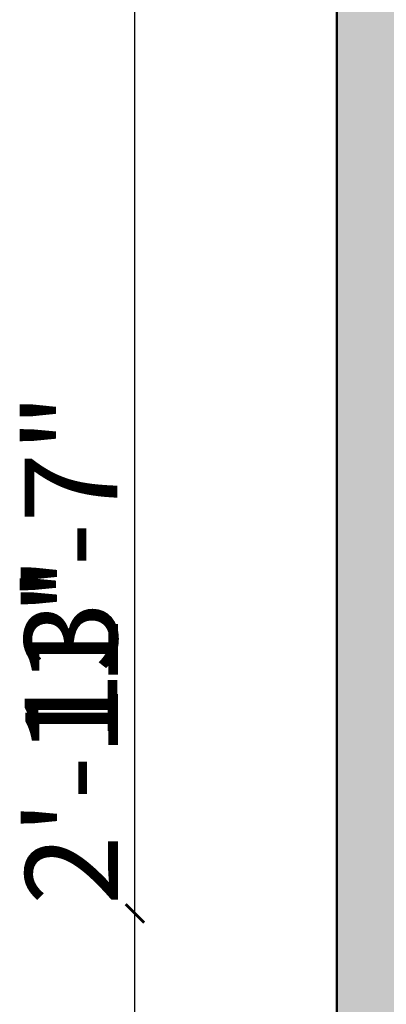
# Model space of a CAD drawing. Units: inches. Extents: x 2419 to 2878, y 1068 to 1713.
# Tile 1 of 20: x 2429 to 2478, y 1153 to 1286. Entities that reach past the tile are written whole.
import ezdxf

# ---------------------------------------------------------------- set-up
doc = ezdxf.new("R2010")
doc.units = ezdxf.units.IN
doc.layers.add('A-ANNO-DIMS', color=2, linetype='Continuous', lineweight=18)
doc.layers.add('A-WALL', color=7, linetype='Continuous', lineweight=50)
doc.layers.add('A-WALL-PATT', color=18, linetype='Continuous', lineweight=13, true_color=0x000000)
doc.styles.get("Standard").update_dxf_attribs({"font": 'arial.ttf'})
doc.dimstyles.new('ISO-25', dxfattribs={"dimtxt": 12.5, "dimasz": 2.5, "dimexe": 1.25, "dimexo": 0.625, "dimtad": 1, "dimdec": 0, "dimlunit": 4, "dimtxsty": 'Standard', "dimblk": 'ARCHTICK', "dimcen": 2.5, "dimse1": 1, "dimse2": 1, "dimclrd": 4, "dimadec": 0, "dimazin": 0, "dimtfac": 1, "dimtdec": 0, "dimtmove": 0, "dimatfit": 3, "dimfxl": 1, "dimarcsym": 0})

# ---------------------------------------------------------------- blocks, each defined once
blk = doc.blocks.new('_ArchTick')
at = {"color": 0, "linetype": 'ByBlock', "const_width": 0.15}
blk.add_lwpolyline([(-0.5, -0.5), (0.5, 0.5)], dxfattribs=at)
blk = doc.blocks.new('*D38')
at = {"layer": 'A-ANNO-DIMS', "color": 4, "lineweight": -2, "transparency": 16777216}
for p, q in [((2444.314464000002, 1165.602617), (2444.314464000002, 1212.505754789905)), ((2444.314464000002, 1130.812987), (2444.314464000002, 1165.602617))]:
    blk.add_line(p, q, dxfattribs=at)
at = {"layer": 'Defpoints', "color": 0, "transparency": 16777216}
for p in [(2444.314464000002, 1165.602617), (2656.740829000001, 1165.602617), (2656.740829000001, 1130.812987)]:
    blk.add_point(p, dxfattribs=at)
at = {"layer": 'A-ANNO-DIMS', "color": 4, "lineweight": -2, "transparency": 16777216, "xscale": 2.5, "yscale": 2.5, "zscale": 2.5}
for p, rotation in [((2444.314464000002, 1165.602617), 90), ((2444.314464000002, 1130.812987), 270)]:
    blk.add_blockref('_ArchTick', p, dxfattribs=dict(at, rotation=rotation))
at = {"layer": 'A-ANNO-DIMS', "color": 0, "transparency": 16777216, "insert": (2437.413884190998, 1190.304185894951), "char_height": 12.5, "attachment_point": 5, "rotation": 90}
blk.add_mtext('2\'-11"', dxfattribs=at)
blk = doc.blocks.new('*D54')
at = {"layer": 'A-ANNO-DIMS', "color": 4, "lineweight": -2, "transparency": 16777216}
blk.add_line((2444.314464000002, 1130.812987), (2444.314464000002, 1293.812987), dxfattribs=at)
at = {"layer": 'Defpoints', "color": 0, "transparency": 16777216}
for p in [(2444.314464000002, 1293.812987), (2480.514464000001, 1293.812987), (2480.514464000001, 1130.812987)]:
    blk.add_point(p, dxfattribs=at)
at = {"layer": 'A-ANNO-DIMS', "color": 4, "lineweight": -2, "transparency": 16777216, "xscale": 2.5, "yscale": 2.5, "zscale": 2.5}
for p, rotation in [((2444.314464000002, 1293.812987), 90), ((2444.314464000002, 1130.812987), 270)]:
    blk.add_blockref('_ArchTick', p, dxfattribs=dict(at, rotation=rotation))
at = {"layer": 'A-ANNO-DIMS', "color": 0, "transparency": 16777216, "insert": (2437.30303835198, 1212.312987), "char_height": 12.5, "attachment_point": 5, "rotation": 90}
blk.add_mtext('13\'-7"', dxfattribs=at)

msp = doc.modelspace()

# ---------------------------------------------------------------- hatches: boundary and pattern name
at = {"layer": 'A-WALL-PATT'}
h = msp.add_hatch(color=256, dxfattribs=at)
h.dxf.hatch_style = 1
h.paths.add_polyline_path([(2780.514463761465, 1577.812987234935), (2471.514463761465, 1577.812987234935), (2471.514463761465, 1121.812987234935), (2780.514463761465, 1121.812987234935)])
h.paths.add_polyline_path([(2480.514463761465, 1568.812987234935), (2771.514463761465, 1568.812987234935), (2771.514463761465, 1130.812987234935), (2480.514463761465, 1130.812987234935)], flags=16)
h.paths.add_polyline_path([(2528.514463761465, 1568.812987234935), (2528.514463761465, 1512.812987234935), (2594.514463761465, 1512.812987234935), (2594.514463761465, 1414.812987234935), (2596.568399739099, 1414.812987234935), (2596.568399739099, 1441.609368546496), (2597.816088158561, 1441.609368546496), (2597.816088158561, 1441.582062289591, -0.38401605427067), (2625.03494332709, 1414.812987234935), (2725.514463761465, 1414.812987234935), (2725.514463761465, 1567.54501314674), (2728.302225194595, 1567.54501314674), (2746.887301415459, 1567.54501314674), (2746.887301415459, 1566.731916062077), (2746.869506397459, 1566.731916062077, -0.3672161804255682), (2730.514463761465, 1549.092071412193), (2730.514463761465, 1512.812987234935), (2750.853045566032, 1512.812987234935), (2750.853045566032, 1510.025225801806, -0.4014527144963593), (2733.081066429831, 1491.457944598941), (2733.081066429831, 1491.440149580942), (2732.267969345168, 1491.440149580942), (2732.267969345168, 1507.812987234935), (2730.514463761465, 1507.812987234935), (2730.514463761465, 1408.812987234935), (2736.514463761465, 1408.812987234935), (2736.514463761466, 1349.812987234935), (2632.514463761465, 1349.812987234935), (2632.514463761465, 1408.812987234935), (2528.514463761465, 1408.812987234935), (2528.514463761465, 1414.812987234935), (2503.967100522841, 1414.812987234935), (2503.967100522841, 1494.852151014206), (2558.37888418044, 1494.852151014206), (2558.37888418044, 1507.812987234935), (2529.964934876797, 1507.812987234936, -0.4142135623730951), (2530.820819834016, 1506.957102277716), (2530.820819834016, 1497.257075044924, -0.4142135623730951), (2529.964934876797, 1496.401190087705), (2514.55900564685, 1496.401190087705, -0.4142135623730903), (2513.703120689631, 1497.257075044924), (2513.703120689631, 1506.957102277716, -0.4142135623730951), (2514.55900564685, 1507.812987234936), (2528.514463761465, 1507.812987234936), (2528.514463761465, 1512.812987234935), (2480.514463761465, 1512.812987234935)], flags=0)
h.paths.add_polyline_path([(2516.261971761824, 1507.812987234935), (2528.261968761824, 1507.812987234935), (2528.261968761824, 1505.812987234935), (2523.416669079506, 1505.812987234935), (2524.073835609436, 1504.674744674158), (2529.394344905318, 1504.674744674158, -0.4142135623730951), (2529.964934876797, 1504.104154702678), (2529.964934876797, 1497.827665016404, -0.4142135623730951), (2529.394344905318, 1497.257075044924), (2515.12959561833, 1497.257075044924, -0.4142135623730987), (2514.55900564685, 1497.827665016404), (2514.55900564685, 1504.104154702678, -0.4142135623730951), (2515.12959561833, 1504.674744674158), (2520.688784298745, 1504.674744674158), (2521.342314766239, 1505.812987234935), (2516.261971761824, 1505.812987234935)], flags=0)
h.paths.add_polyline_path([(2522.015649482737, 1505.530629631377), (2522.816542912466, 1507.317910507759, -0.6550601971121365), (2522.254220692544, 1506.063027257721), (2522.194533044389, 1505.929827773067), (2522.425009080837, 1505.530629631377)], flags=0)
h.paths.add_polyline_path([(2522.832560233303, 1500.965909859541, -1), (2521.691380290344, 1500.965909859541, -1)], flags=0)
h.paths.add_polyline_path([(2522.547265247564, 1500.965909859541, -1), (2521.976675276084, 1500.965909859541, -1)], flags=0)
h.paths.add_polyline_path([(2482.005175746464, 1470.632511127513), (2499.893716585039, 1470.632511127513), (2499.893716585039, 1448.271831352515), (2482.005175746464, 1448.271831352515), (2482.005175746464, 1452.743967307515), (2481.259819753965, 1452.743967307515), (2481.259819753965, 1449.762543337515), (2480.514463761465, 1449.762543337515), (2480.514463761465, 1469.141799142513), (2481.259819753965, 1469.141799142513), (2481.259819753965, 1466.160375172514), (2482.005175746464, 1466.160375172514)], flags=0)
h.paths.add_polyline_path([(2488.71337669754, 1466.160375172514, -1), (2484.24124074254, 1466.160375172514, -1)], flags=0)
h.paths.add_polyline_path([(2496.166936473468, 1466.160375172514, -1), (2490.204088533468, 1466.160375172514, -1)], flags=0)
h.paths.add_polyline_path([(2487.96802070504, 1466.160375172514, -1), (2484.986596735041, 1466.160375172514, -1)], flags=0)
h.paths.add_polyline_path([(2495.421580480968, 1466.160375172514, -1), (2490.949444525969, 1466.160375172514, -1)], flags=0)
h.paths.add_polyline_path([(2487.22266471254, 1466.160375172514, -1), (2485.731952727541, 1466.160375172514, -1)], flags=0)
h.paths.add_polyline_path([(2494.676224488468, 1466.160375172514, -1), (2491.694800518468, 1466.160375172514, -1)], flags=0)
h.paths.add_polyline_path([(2499.10799430668, 1468.004897240262, -1), (2497.977225324558, 1468.004897240262, -1)], flags=0)
h.paths.add_polyline_path([(2493.930868495968, 1466.160375172514, -1), (2492.440156510968, 1466.160375172514, -1)], flags=0)
h.paths.add_polyline_path([(2499.37156767049, 1463.70992381177, -1), (2498.1659645309, 1463.70992381177, -1)], flags=0)
h.paths.add_polyline_path([(2484.241243723964, 1461.688239217514), (2496.16693662254, 1461.688239217514), (2496.16693662254, 1457.216103262515), (2484.241243723964, 1457.216103262515)], flags=0)
h.paths.add_polyline_path([(2484.986599716464, 1460.942883225014), (2495.42158063004, 1460.942883225014), (2495.42158063004, 1457.961459255015), (2484.986599716464, 1457.961459255015)], flags=0)
h.paths.add_polyline_path([(2586.879843577569, 1510.025225801806), (2587.692940662232, 1510.025225801806), (2587.692940662232, 1491.440149580942), (2586.879843577569, 1491.440149580942)], flags=0)
h.paths.add_polyline_path([(2499.258769311151, 1459.414950383278, -1), (2498.203381609636, 1459.414950383278, -1)], flags=0)
h.paths.add_polyline_path([(2489.45873269004, 1452.743967307515, -1), (2483.49588475004, 1452.743967307515, -1)], flags=0)
h.paths.add_polyline_path([(2557.29940140061, 1408.812987234935), (2557.29940140061, 1413.090776101661, -0.4014527144963548), (2584.570305425984, 1441.582062289591), (2584.570305425984, 1441.609368546496), (2585.817993845445, 1441.609368546496), (2585.817993845445, 1413.090776101661), (2585.817993845445, 1408.812987234935)], flags=0)
h.paths.add_polyline_path([(2488.71337669754, 1452.743967307515, -1), (2484.24124074254, 1452.743967307515, -1)], flags=0)
h.paths.add_polyline_path([(2495.421580480968, 1452.743967307515, -1), (2490.949444525969, 1452.743967307515, -1)], flags=0)
h.paths.add_polyline_path([(2487.96802070504, 1452.743967307515, -1), (2484.986596735041, 1452.743967307515, -1)], flags=0)
h.paths.add_polyline_path([(2494.676224488468, 1452.743967307515, -1), (2491.694800518468, 1452.743967307515, -1)], flags=0)
h.paths.add_polyline_path([(2487.22266471254, 1452.743967307515, -1), (2485.731952727541, 1452.743967307515, -1)], flags=0)
h.paths.add_polyline_path([(2499.18308934039, 1454.441826005015, -1), (2497.902130290848, 1454.441826005015, -1)], flags=0)
h.paths.add_polyline_path([(2493.930868495968, 1452.743967307515, -1), (2492.440156510968, 1452.743967307515, -1)], flags=0)
h.paths.add_polyline_path([(2499.296459951454, 1450.636626811365, -1), (2497.788759679783, 1450.636626811365, -1)], flags=0)
h.paths.add_polyline_path([(2619.128766651402, 1558.889032727177, -1), (2605.128766651402, 1558.889032727177, -1)], flags=0)
h.paths.add_polyline_path([(2609.128766651402, 1558.889032727177), (2612.128766651402, 1561.889033727177), (2615.128769651402, 1558.889032727177), (2612.128766651402, 1555.889032727177)], flags=0)
h.paths.add_polyline_path([(2611.128766651402, 1558.889032727177, -1), (2613.128766651402, 1558.889032727177, -1)], flags=0)
h.paths.add_polyline_path([(2633.678910285153, 1568.812987234935), (2693.678900285153, 1568.812987234935), (2693.678900285153, 1488.812957234935), (2633.678910285153, 1488.812957234935)], flags=0)
h.paths.add_polyline_path([(2641.678900285152, 1554.412987234935), (2641.678900285152, 1567.612987234935), (2662.478890285152, 1567.612987234935), (2662.478890285152, 1554.412987234935), (2664.878900285153, 1554.412987234935), (2664.878900285153, 1567.612987234935), (2685.678900285152, 1567.612987234935), (2685.678900285152, 1552.412987234935), (2680.478908969363, 1552.412987234935), (2693.678900285153, 1539.212987234935), (2678.478910285153, 1539.212987234935), (2678.478910285153, 1554.412987234935)], flags=0)
h.paths.add_polyline_path([(2637.514463761465, 1408.812987234935), (2731.514463761465, 1408.812987234935), (2731.514463761465, 1354.812987234935), (2637.514463761465, 1354.812987234935), (2637.514463761465, 1357.97634876414), (2635.302225194595, 1357.97634876414), (2635.302225194595, 1358.789445848803), (2637.514463761465, 1358.789445848803)], flags=0)
h.paths.add_polyline_path([(2717.171392308236, 1559.642859555671, -1), (2703.171392308235, 1559.642859555671, -1)], flags=0)
h.paths.add_polyline_path([(2707.171392308235, 1559.642859555671), (2710.171392308236, 1562.642860555671), (2713.171395308235, 1559.642859555671), (2710.171392308236, 1556.642859555671)], flags=0)
h.paths.add_polyline_path([(2709.171392308235, 1559.642859555671, -1), (2711.171392308235, 1559.642859555671, -1)], flags=0)
h.paths.add_polyline_path([(2685.37839484874, 1408.812987234935), (2706.37839484874, 1408.812987234935), (2706.37839484874, 1400.812987234935), (2699.87839484874, 1400.812987234935), (2701.8783582045, 1394.813097167654, -0.5013234908365424), (2696.923094014159, 1375.951847407521, -0.1328909081880473), (2694.833737505469, 1375.951847423997, -0.5013167773010871), (2689.878359877304, 1394.812882320626), (2691.87839484874, 1400.812987234935), (2688.87839484874, 1400.812987234935), (2688.87839484874, 1399.312987234935), (2685.87839484874, 1399.312987234935), (2685.87839484874, 1400.312987234935), (2687.87839484874, 1400.312987234935), (2687.87839484874, 1400.812987234935), (2685.37839484874, 1400.812987234935)], flags=0)
h.paths.add_polyline_path([(2687.378395015029, 1407.812987234935), (2704.37839468245, 1407.812987234935, -0.5000001164019596), (2705.37839484874, 1406.812987068648), (2705.37839484874, 1402.812987401223, -0.5000001164019594), (2704.37839468245, 1401.812987234935), (2687.378395015029, 1401.812987234935, -0.5000001164019899), (2686.37839484874, 1402.812987401223), (2686.37839484874, 1406.812987068648, -0.5000001164019594)], flags=0)
h.paths.add_polyline_path([(2639.514463761465, 1205.812987234935), (2634.514463761465, 1205.812987234935), (2634.514463761464, 1293.812987234935), (2637.514463761466, 1293.812987234935), (2639.514463761465, 1293.812987234935)], flags=0)
h.paths.add_polyline_path([(2691.878449271624, 1394.812987234935), (2699.878439365793, 1394.812987234935, -0.4800795019661124), (2697.522447975332, 1377.289995604548, -0.2150037826744892), (2694.234383577574, 1377.28999563916, -0.4800796505540576)], flags=0)
h.paths.add_polyline_path([(2757.514358847156, 1453.891486469081), (2763.514463761465, 1451.891451497645), (2763.514463761465, 1454.891451497645), (2762.014463761465, 1454.891451497645), (2762.014463761465, 1457.891451497645), (2763.014463761465, 1457.891451497645), (2763.014463761465, 1455.891451497645), (2763.514463761465, 1455.891451497645), (2763.514463761465, 1458.391451497645), (2771.514463761465, 1458.391451497645), (2771.514463761465, 1437.391451497645), (2763.514463761465, 1437.391451497645), (2763.514463761465, 1443.891451497645), (2757.514573694182, 1441.891488141884, -0.5013234908367097), (2738.653323934048, 1446.846752332236, -0.1328909081861904), (2738.653323950519, 1448.936108840897, -0.5013167773016524)], flags=0)
h.paths.add_polyline_path([(2739.991472165689, 1449.535462768808, -0.4800796505541595), (2757.514463761465, 1451.891397074762), (2757.514463761465, 1443.891406980593, -0.4800795019659427), (2739.991472131081, 1446.247398371048, -0.2150037826747098)], flags=0)
h.paths.add_polyline_path([(2765.514463927754, 1457.391451497645), (2769.514463595176, 1457.391451497645, -0.500000116401859), (2770.514463761465, 1456.391451331358), (2770.514463761465, 1439.391451663933, -0.500000116401859), (2769.514463595176, 1438.391451497645), (2765.514463927754, 1438.391451497645, -0.500000116401859), (2764.514463761465, 1439.391451663933), (2764.514463761465, 1456.391451331358, -0.5000001164020391)], flags=0)

# ---------------------------------------------------------------- linework, layer by layer
at = {"layer": 'A-WALL'}
msp.add_lwpolyline([(2471.514463761465, 1577.812987234935), (2780.514463761465, 1577.812987234935), (2780.514463761465, 1121.812987234935), (2471.514463761465, 1121.812987234935)], close=True, dxfattribs=at)

# ---------------------------------------------------------------- dimensions: what is measured, and where the dimension line sits
at = {"layer": 'A-ANNO-DIMS'}
for base, p1, p2, picture, middle in [((2444.314464000002, 1293.812987), (2480.514464, 1130.812987), (2480.514464, 1293.812987), '*D54', (2437.30303835198, 1212.312987)), ((2444.314464000002, 1165.602617), (2656.740829, 1130.812987), (2656.740829, 1165.602617), '*D38', (2437.413884190998, 1190.304185894951))]:
    dim = msp.add_linear_dim(base=base, p1=p1, p2=p2, angle=90, dimstyle='ISO-25', override={"dimdec": 1, "dimlfac": 1, "dimrnd": 0, "dimzin": 1, "dimdsep": 46, "dimlunit": 4, "dimfrac": 2}, dxfattribs=at)
    dim.commit()
    dim.dimension.update_dxf_attribs({"geometry": picture, "text_midpoint": middle})

doc.saveas('drawing.dxf')
